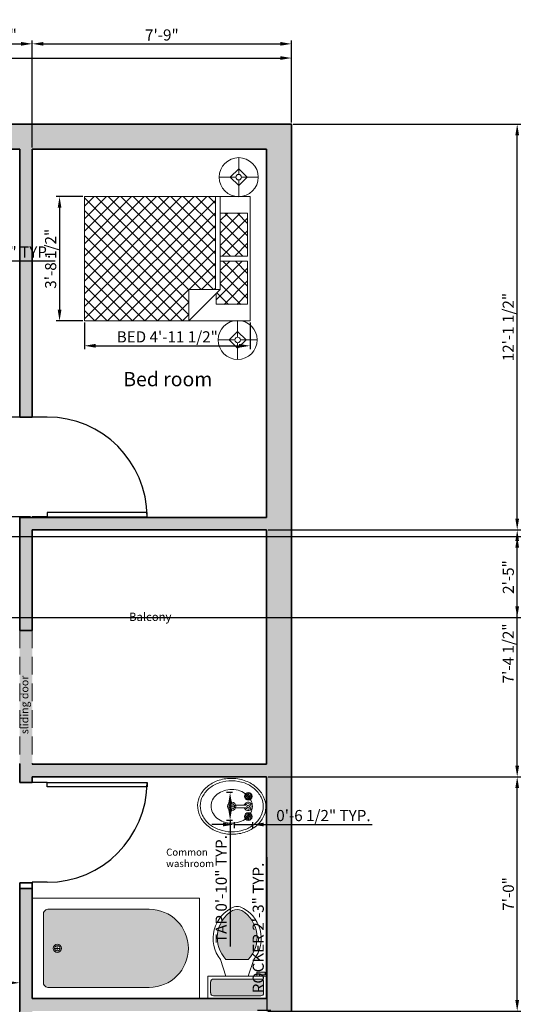
# Model space of a CAD drawing. Units: inches. Extents: x 1872 to 2380, y 714 to 1327.
# Tile 9 of 9: x 2198 to 2380, y 974 to 1327. Entities that reach past the tile are written whole.
import ezdxf

# ---------------------------------------------------------------- set-up
doc = ezdxf.new("R2010")
doc.units = ezdxf.units.IN
doc.linetypes.add('HIDDEN', pattern=[9.525, 6.35, -3.175])
for name, color, linetype, lineweight in [('A-ANNO-DIMS', 2, 'Continuous', 18), ('A-ANNO-TEXT', 7, 'Continuous', 18), ('A-AREA-IDEN', 7, 'Continuous', 18), ('A-DOOR', 4, 'Continuous', 25), ('A-DOOR-HIDN', 4, 'HIDDEN', 18), ('A-FLOR-FIXT', 9, 'Continuous', 20), ('A-FURN', 8, 'Continuous', 18), ('A-WALL', 7, 'Continuous', 35)]:
    doc.layers.add(name, color=color, linetype=linetype, lineweight=lineweight)
for name, color, linetype, lineweight, true_color in [('A-FLOR-FIXT-PATT', 7, 'Continuous', 13, 0xd1ffff), ('A-FURN-PATT', 254, 'Continuous', 13, 0xf8ceb3), ('A-WALL-PATT', 242, 'Continuous', 13, 0xd52e31)]:
    doc.layers.add(name, color=color, linetype=linetype, lineweight=lineweight, true_color=true_color)
doc.styles.get("Standard").update_dxf_attribs({"font": 'arial.ttf'})
doc.dimstyles.new('ISO-25', dxfattribs={"dimtxt": 4, "dimasz": 4, "dimexe": 1.25, "dimexo": 0.625, "dimtad": 1, "dimdec": 0, "dimlunit": 3, "dimtxsty": 'Standard', "dimcen": 2.5, "dimadec": 0, "dimazin": 0, "dimtfac": 1, "dimtdec": 0, "dimtmove": 0, "dimatfit": 3, "dimfxl": 1, "dimarcsym": 0})

# ---------------------------------------------------------------- blocks, each defined once
blk = doc.blocks.new('*U4')
for p, q in [((0, 0), (0, -6)), ((-40, 0), (-40, -6))]:
    blk.add_line(p, q)
blk.add_lwpolyline([(0, 0), (0, 40), (-1.75, 40), (-1.75, 0)], close=True)
blk.add_arc((0, 0), 40, 90, 180)
blk = doc.blocks.new('*U3')
for p, q in [((0, 0), (0, -6)), ((40, 0), (40, -6))]:
    blk.add_line(p, q)
blk.add_lwpolyline([(0, 0), (0, 40), (1.75, 40), (1.75, 0)], close=True)
blk.add_arc((0, 0), 40, 0, 90)
blk = doc.blocks.new('Bed - Queen')
for p, q in [((0, -80.00003), (0, 0)), ((0, 0), (59.99999, 0)), ((59.99999, 0), (59.99999, -80.00003)), ((7.99999, -1.2), (28.79998, -1.2)), ((7.99999, -14.4), (7.99999, -1.2)), ((28.79998, -1.2), (28.79998, -14.4)), ((31.19999, -1.2), (51.99999, -1.2)), ((31.19999, -14.4), (31.19999, -1.2)), ((51.99999, -1.2), (51.99999, -16.4)), ((0, -14.4), (44.8, -14.4)), ((44.8, -16.8), (0, -16.8)), ((59.99999, -29.6), (44.8, -14.4)), ((44.8, -14.4), (44.8, -29.6)), ((51.99999, -16.4), (46.79936, -16.4)), ((44.8, -29.6), (59.99999, -29.6)), ((59.99999, -80.00003), (0, -80.00003))]:
    blk.add_line(p, q)
blk = doc.blocks.new('Lamp - Table')
for p, q in [((0, 7), (0, 1)), ((-1, 0), (-7, 0)), ((0, 3), (-3, 0)), ((-3, 0), (0, -3)), ((3, 0), (0, 3)), ((0, -3), (3, 0)), ((1, 0), (7, 0)), ((0, -1), (0, -7))]:
    blk.add_line(p, q)
for radius in [7, 1]:
    blk.add_circle((0, 0), radius)
blk = doc.blocks.new('Toilet - top')
for p, q in [((9.5, -6), (9.5, -2)), ((-10, -8.5), (-8, -8.5)), ((-10, -9.5), (-10, -8.5)), ((-7, -9.5), (-10, -9.5)), ((-8, -8.5), (-8, -8)), ((-7, -8), (-7, -9.5)), ((-4, -8), (-6, -14)), ((4, -8), (6, -14)), ((4, -14), (-4, -14))]:
    blk.add_line(p, q)
blk.add_lwpolyline([(10.5, -8), (10.5, 0), (-10.5, 0), (-10.5, -8)], close=True)
for points in [[(-9.5, -2), (-9.5, -6)], [(8.5, -1), (-8.5, -1)], [(-8.5, -7), (8.5, -7)]]:
    blk.add_lwpolyline(points)
for centre, radius, start, end in [((-8.62, -1.88), 0.884, 81.8699, 188.1301), ((8.62, -1.88), 0.884, 351.8699, 98.1301), ((-8.62, -6.12), 0.884, 171.8699, 278.1301), ((8.62, -6.12), 0.884, 261.8699, 8.1301), ((3.52, -21.58), 12.17, 141.4691, 247.9714), ((4.2, -21.82), 11.33, 136.3677, 238.9468), ((-3.52, -21.58), 12.17, 292.0284, 38.5307), ((-4.2, -21.82), 11.33, 301.053, 43.6321), ((0, -27.88), 4, 245.7318, 294.2682), ((0, -29), 4, 254.8605, 285.1395)]:
    blk.add_arc(centre, radius, start, end)
blk = doc.blocks.new('Bath Tub - 26 x 60 in.')
for p, q in [((9, -17), (9, -19)), ((8, -18), (10, -18))]:
    blk.add_line(p, q)
blk.add_lwpolyline([(0, -36), (0, 0), (60, 0), (60, -36)], close=True)
for points in [[(4, -30), (4, -6)], [(6, -4), (42, -4)], [(42, -32), (6, -32)]]:
    blk.add_lwpolyline(points)
for radius in [1.5, 1]:
    blk.add_circle((9, -18), radius)
for centre, radius, start, end in [((5.75, -5.75), 1.77, 81.8699, 188.1301), ((42, -18), 14, 270, 90), ((5.75, -30.25), 1.77, 171.8699, 278.1301)]:
    blk.add_arc(centre, radius, start, end)
blk = doc.blocks.new('Sink - Oval top')
for p, q in [((-1, 0), (1, 0)), ((0, 1), (0, -1))]:
    blk.add_line(p, q)
for points in [[(-12.23, 0.39, 0.117634), (-11.46, -3.36, 0.104469), (-8.88, -6.8, 0.090016), (-5.08, -9.07, 0.08192), (-0.32, -10.02, 0.08192), (4.49, -9.38, 0.090016), (8.42, -7.36, 0.104469), (11.22, -4.09, 0.117634), (12.23, -0.39, 0.117634), (11.46, 3.36, 0.104469), (8.88, 6.8, 0.090016), (5.08, 9.07, 0.08192), (0.32, 10.02, 0.08192), (-4.49, 9.38, 0.090016), (-8.42, 7.36, 0.104469), (-11.22, 4.09, 0.117634)], [(-11.29, 0.16, 0.118622), (-10.52, -3.25, 0.104678), (-8.07, -6.36, 0.089562), (-4.54, -8.37, 0.081185), (-0.13, -9.15, 0.081185), (4.3, -8.49, 0.089562), (7.89, -6.58, 0.104678), (10.42, -3.55, 0.118622), (11.29, -0.16, 0.118622), (10.52, 3.25, 0.104678), (8.07, 6.36, 0.089562), (4.54, 8.37, 0.081185), (0.13, 9.15, 0.081185), (-4.3, 8.49, 0.089562), (-7.89, 6.58, 0.104678), (-10.42, 3.55, 0.118622)], [(-7.42, 0.08, 0.118283), (-6.91, -2.17, 0.104607), (-5.29, -4.21, 0.089718), (-2.97, -5.53, 0.081436), (-0.07, -6.04, 0.081436), (2.84, -5.59, 0.089718), (5.2, -4.33, 0.104607), (6.86, -2.32, 0.118283), (7.42, -0.08, 0.118283), (6.91, 2.17, 0.104607), (5.29, 4.21, 0.089718), (2.97, 5.53, 0.081436), (0.07, 6.04, 0.081436), (-2.84, 5.59, 0.089718), (-5.2, 4.33, 0.104607), (-6.86, 2.32, 0.118283)]]:
    blk.add_lwpolyline(points, format="xyb", close=True)
for radius in [1.5, 1]:
    blk.add_circle((0, 0), radius)
blk = doc.blocks.new('Faucet - Bathroom top')
for p, q in [((-4.107, 0.125), (-4.375, 0.125)), ((-3.75, 0.4788), (-3.75, 0.75)), ((-3.5, 0.482), (-3.5, 0.75)), ((-3.1461, 0.125), (-2.875, 0.125)), ((3.143, 0.125), (2.875, 0.125)), ((3.5, 0.4788), (3.5, 0.75)), ((3.75, 0.482), (3.75, 0.75)), ((4.1039, 0.125), (4.375, 0.125)), ((-4.1039, -0.125), (-4.375, -0.125)), ((-3.75, -0.4821), (-3.75, -0.75)), ((-3.5, -0.4789), (-3.5, -0.75)), ((-3.143, -0.125), (-2.875, -0.125)), ((-0.5, -0.8639), (-0.5, -4.5)), ((0.5, -4.5), (0.5, -0.8631)), ((3.1461, -0.125), (2.875, -0.125)), ((3.5, -0.4821), (3.5, -0.75)), ((3.75, -0.4789), (3.75, -0.75)), ((4.107, -0.125), (4.375, -0.125))]:
    blk.add_line(p, q)
for centre, radius in [((-3.625, 0), 1.375), ((-4.625, 0), 0.2795), ((-3.625, 0), 0.5), ((-3.625, 1), 0.2795), ((-2.625, 0), 0.2795), ((0, 0), 0.5), ((3.625, 0), 1.375), ((2.625, 0), 0.2795), ((3.625, 0), 0.5), ((3.625, 1), 0.2795), ((4.625, 0), 0.2795), ((-3.625, -1), 0.2795), ((3.625, -1), 0.2795)]:
    blk.add_circle(centre, radius)
for centre, radius, start, end in [((-3.625, 0), 1, 105.2407, 164.2093), ((-3.625, 0), 1, 16.44125, 74.07887), ((0, 0), 1.5, 289.6514, 250.3603), ((0, 0), 1, 300.3431, 239.7554), ((3.625, 0), 1, 106.12, 164.0884), ((3.625, 0), 1, 16.23422, 73.90469), ((-3.625, 0), 1, 196.2342, 253.9047), ((-3.625, 0), 1, 286.12, 344.0884), ((3.625, 0), 1, 196.4413, 254.0789), ((3.625, 0), 1, 285.2407, 344.2093), ((0, -4.5), 0.5, 180, 0)]:
    blk.add_arc(centre, radius, start, end)
blk = doc.blocks.new('*D22')
at = {"layer": 'A-ANNO-DIMS', "color": 0, "lineweight": -2, "transparency": 16777216}
for p, q in [((1935.4, 1290.27), (1935.4, 1314.61)), ((1939.4, 1313.36), (2291.4, 1313.36)), ((2295.4, 1290.27), (2295.4, 1314.61))]:
    blk.add_line(p, q, dxfattribs=at)
at = {"layer": 'A-ANNO-DIMS', "color": 0, "transparency": 16777216}
for points in [[(1939.4, 1314.03), (1939.4, 1312.69), (1935.4, 1313.36)], [(2291.4, 1314.03), (2291.4, 1312.69), (2295.4, 1313.36)]]:
    blk.add_solid(points, dxfattribs=at)
at = {"layer": 'Defpoints', "color": 0, "transparency": 16777216}
for p in [(2295.4, 1313.36), (1935.4, 1289.64), (2295.4, 1289.64)]:
    blk.add_point(p, dxfattribs=at)
at = {"layer": 'A-ANNO-DIMS', "color": 0, "transparency": 16777216, "insert": (2115.4, 1316.03), "char_height": 4, "attachment_point": 5}
blk.add_mtext("30'", dxfattribs=at)
blk = doc.blocks.new('*D28')
at = {"layer": 'A-ANNO-DIMS', "color": 0, "lineweight": -2, "transparency": 16777216}
for p, q in [((2221.12, 1218.47), (2221.12, 1208.93)), ((2280.56, 1218.47), (2280.56, 1208.93)), ((2225.12, 1210.18), (2276.56, 1210.18))]:
    blk.add_line(p, q, dxfattribs=at)
at = {"layer": 'A-ANNO-DIMS', "color": 0, "transparency": 16777216}
for points in [[(2225.12, 1210.85), (2225.12, 1209.51), (2221.12, 1210.18)], [(2276.56, 1210.85), (2276.56, 1209.51), (2280.56, 1210.18)]]:
    blk.add_solid(points, dxfattribs=at)
at = {"layer": 'Defpoints', "color": 0, "transparency": 16777216}
for p in [(2221.12, 1219.09), (2280.56, 1219.09), (2280.56, 1210.18)]:
    blk.add_point(p, dxfattribs=at)
at = {"layer": 'A-ANNO-DIMS', "color": 0, "transparency": 16777216, "insert": (2250.84, 1212.87), "char_height": 4, "attachment_point": 5}
blk.add_mtext('BED 4\'-11 1/2"', dxfattribs=at)
blk = doc.blocks.new('*D29')
at = {"layer": 'A-ANNO-DIMS', "color": 0, "lineweight": -2, "transparency": 16777216}
for p, q in [((2220.5, 1263.68), (2210.95, 1263.68)), ((2212.2, 1259.68), (2212.2, 1223.09)), ((2220.5, 1219.09), (2210.95, 1219.09))]:
    blk.add_line(p, q, dxfattribs=at)
at = {"layer": 'A-ANNO-DIMS', "color": 0, "transparency": 16777216}
for points in [[(2211.54, 1259.68), (2212.87, 1259.68), (2212.2, 1263.68)], [(2211.54, 1223.09), (2212.87, 1223.09), (2212.2, 1219.09)]]:
    blk.add_solid(points, dxfattribs=at)
at = {"layer": 'Defpoints', "color": 0, "transparency": 16777216}
for p in [(2221.12, 1263.68), (2212.2, 1219.09), (2221.12, 1219.09)]:
    blk.add_point(p, dxfattribs=at)
at = {"layer": 'A-ANNO-DIMS', "color": 0, "transparency": 16777216, "insert": (2209.51, 1241.38), "char_height": 4, "attachment_point": 5, "rotation": 90}
blk.add_mtext('3\'-8 1/2"', dxfattribs=at)
blk = doc.blocks.new('*D32')
at = {"layer": 'A-ANNO-DIMS', "color": 0, "lineweight": -2, "transparency": 16777216}
for p, q in [((2274.25, 1050.03), (2272.12, 1050.03)), ((2273.37, 1046.03), (2273.37, 1044.03)), ((2274.25, 1040.03), (2272.12, 1040.03)), ((2273.37, 1040.03), (2273.37, 994.77))]:
    blk.add_line(p, q, dxfattribs=at)
at = {"layer": 'A-ANNO-DIMS', "color": 0, "transparency": 16777216}
for points in [[(2272.7, 1046.03), (2274.04, 1046.03), (2273.37, 1050.03)], [(2272.7, 1044.03), (2274.04, 1044.03), (2273.37, 1040.03)]]:
    blk.add_solid(points, dxfattribs=at)
at = {"layer": 'Defpoints', "color": 0, "transparency": 16777216}
for p in [(2274.87, 1050.03), (2273.37, 1040.03), (2274.87, 1040.03)]:
    blk.add_point(p, dxfattribs=at)
at = {"layer": 'A-ANNO-DIMS', "color": 0, "transparency": 16777216, "insert": (2270.7, 1015.4), "char_height": 4, "attachment_point": 5, "rotation": 90}
blk.add_mtext('TAP 0\'-10" TYP.', dxfattribs=at)
blk = doc.blocks.new('*D33')
at = {"layer": 'A-ANNO-DIMS', "color": 0, "lineweight": -2, "transparency": 16777216}
for p, q in [((2270.87, 1038.53), (2266.87, 1038.53)), ((2274.87, 1039.41), (2274.87, 1037.28)), ((2274.87, 1038.53), (2281.37, 1038.53)), ((2281.37, 1039.41), (2281.37, 1037.28)), ((2285.37, 1038.53), (2324.32, 1038.53))]:
    blk.add_line(p, q, dxfattribs=at)
at = {"layer": 'A-ANNO-DIMS', "color": 0, "transparency": 16777216}
for points in [[(2270.87, 1039.2), (2270.87, 1037.87), (2274.87, 1038.53)], [(2285.37, 1039.2), (2285.37, 1037.87), (2281.37, 1038.53)]]:
    blk.add_solid(points, dxfattribs=at)
at = {"layer": 'Defpoints', "color": 0, "transparency": 16777216}
for p in [(2274.87, 1040.03), (2281.37, 1040.03), (2281.37, 1038.53)]:
    blk.add_point(p, dxfattribs=at)
at = {"layer": 'A-ANNO-DIMS', "color": 0, "transparency": 16777216, "insert": (2306.85, 1041.23), "char_height": 4, "attachment_point": 5}
blk.add_mtext('0\'-6 1/2" TYP.', dxfattribs=at)
blk = doc.blocks.new('*D36')
at = {"layer": 'A-ANNO-DIMS', "color": 0, "lineweight": -2, "transparency": 16777216}
for p, q in [((2136.87, 1236.27), (2136.87, 1241.85)), ((2140.87, 1240.6), (2165.91, 1240.6)), ((2169.91, 1236.27), (2169.91, 1241.85)), ((2169.91, 1240.6), (2210.57, 1240.6))]:
    blk.add_line(p, q, dxfattribs=at)
at = {"layer": 'A-ANNO-DIMS', "color": 0, "transparency": 16777216}
for points in [[(2140.87, 1241.27), (2140.87, 1239.93), (2136.87, 1240.6)], [(2165.91, 1241.27), (2165.91, 1239.93), (2169.91, 1240.6)]]:
    blk.add_solid(points, dxfattribs=at)
at = {"layer": 'Defpoints', "color": 0, "transparency": 16777216}
for p in [(2169.91, 1240.6), (2136.87, 1235.64), (2169.91, 1235.64)]:
    blk.add_point(p, dxfattribs=at)
at = {"layer": 'A-ANNO-DIMS', "color": 0, "transparency": 16777216, "insert": (2192.24, 1243.29), "char_height": 4, "attachment_point": 5}
blk.add_mtext('WC 2\'-9" TYP.', dxfattribs=at)
blk = doc.blocks.new('*D38')
at = {"layer": 'A-ANNO-DIMS', "color": 0, "lineweight": -2, "transparency": 16777216}
for p, q in [((2286.68, 972), (2286.68, 1026.88)), ((2283.25, 972), (2287.93, 972)), ((2286.68, 949), (2286.68, 968)), ((2283.25, 945), (2287.93, 945))]:
    blk.add_line(p, q, dxfattribs=at)
at = {"layer": 'A-ANNO-DIMS', "color": 0, "transparency": 16777216}
for points in [[(2286.01, 968), (2287.34, 968), (2286.68, 972)], [(2286.01, 949), (2287.34, 949), (2286.68, 945)]]:
    blk.add_solid(points, dxfattribs=at)
at = {"layer": 'Defpoints', "color": 0, "transparency": 16777216}
for p in [(2282.63, 972), (2286.68, 972), (2282.63, 945)]:
    blk.add_point(p, dxfattribs=at)
at = {"layer": 'A-ANNO-DIMS', "color": 0, "transparency": 16777216, "insert": (2283.98, 1001.44), "char_height": 4, "attachment_point": 5, "rotation": 90}
blk.add_mtext('ROCKER 2\'-3" TYP.', dxfattribs=at)
blk = doc.blocks.new('*D54')
at = {"layer": 'A-ANNO-DIMS', "color": 0, "lineweight": -2, "transparency": 16777216}
for p, q in [((2169.91, 1281.27), (2169.91, 1319.69)), ((2173.91, 1318.44), (2198.4, 1318.44)), ((2202.4, 1281.27), (2202.4, 1319.69))]:
    blk.add_line(p, q, dxfattribs=at)
at = {"layer": 'A-ANNO-DIMS', "color": 0, "transparency": 16777216}
for points in [[(2173.91, 1319.11), (2173.91, 1317.78), (2169.91, 1318.44)], [(2198.4, 1319.11), (2198.4, 1317.78), (2202.4, 1318.44)]]:
    blk.add_solid(points, dxfattribs=at)
at = {"layer": 'Defpoints', "color": 0, "transparency": 16777216}
for p in [(2202.4, 1318.44), (2169.91, 1280.64), (2202.4, 1280.64)]:
    blk.add_point(p, dxfattribs=at)
at = {"layer": 'A-ANNO-DIMS', "color": 0, "transparency": 16777216, "insert": (2186.16, 1321.14), "char_height": 4, "attachment_point": 5}
blk.add_mtext('2\'-8 1/2"', dxfattribs=at)
blk = doc.blocks.new('*D55')
at = {"layer": 'A-ANNO-DIMS', "color": 0, "lineweight": -2, "transparency": 16777216}
for p, q in [((2202.4, 1281.27), (2202.4, 1319.69)), ((2206.4, 1318.44), (2291.4, 1318.44)), ((2295.4, 1290.27), (2295.4, 1319.69))]:
    blk.add_line(p, q, dxfattribs=at)
at = {"layer": 'A-ANNO-DIMS', "color": 0, "transparency": 16777216}
for points in [[(2206.4, 1319.11), (2206.4, 1317.78), (2202.4, 1318.44)], [(2291.4, 1319.11), (2291.4, 1317.78), (2295.4, 1318.44)]]:
    blk.add_solid(points, dxfattribs=at)
at = {"layer": 'Defpoints', "color": 0, "transparency": 16777216}
for p in [(2295.4, 1318.44), (2295.4, 1289.64), (2202.4, 1280.64)]:
    blk.add_point(p, dxfattribs=at)
at = {"layer": 'A-ANNO-DIMS', "color": 0, "transparency": 16777216, "insert": (2248.9, 1321.11), "char_height": 4, "attachment_point": 5}
blk.add_mtext('7\'-9"', dxfattribs=at)
blk = doc.blocks.new('*D63')
at = {"layer": 'A-ANNO-DIMS', "color": 0, "lineweight": -2, "transparency": 16777216}
for p, q in [((2287.02, 1055.64), (2377.6, 1055.64)), ((2376.35, 975.64), (2376.35, 1051.64)), ((2287.02, 971.64), (2377.6, 971.64))]:
    blk.add_line(p, q, dxfattribs=at)
at = {"layer": 'A-ANNO-DIMS', "color": 0, "transparency": 16777216}
for points in [[(2375.68, 1051.64), (2377.01, 1051.64), (2376.35, 1055.64)], [(2375.68, 975.64), (2377.01, 975.64), (2376.35, 971.64)]]:
    blk.add_solid(points, dxfattribs=at)
at = {"layer": 'Defpoints', "color": 0, "transparency": 16777216}
for p in [(2286.4, 1055.64), (2376.35, 1055.64), (2286.4, 971.64)]:
    blk.add_point(p, dxfattribs=at)
at = {"layer": 'A-ANNO-DIMS', "color": 0, "transparency": 16777216, "insert": (2373.68, 1013.64), "char_height": 4, "attachment_point": 5, "rotation": 90}
blk.add_mtext('7\'-0"', dxfattribs=at)
blk = doc.blocks.new('*D64')
at = {"layer": 'A-ANNO-DIMS', "color": 0, "lineweight": -2, "transparency": 16777216}
for p, q in [((2287.02, 1144.14), (2377.6, 1144.14)), ((2376.35, 1059.64), (2376.35, 1140.14)), ((2287.02, 1055.64), (2377.6, 1055.64))]:
    blk.add_line(p, q, dxfattribs=at)
at = {"layer": 'A-ANNO-DIMS', "color": 0, "transparency": 16777216}
for points in [[(2375.68, 1140.14), (2377.01, 1140.14), (2376.35, 1144.14)], [(2375.68, 1059.64), (2377.01, 1059.64), (2376.35, 1055.64)]]:
    blk.add_solid(points, dxfattribs=at)
at = {"layer": 'Defpoints', "color": 0, "transparency": 16777216}
for p in [(2286.4, 1144.14), (2376.35, 1144.14), (2286.4, 1055.64)]:
    blk.add_point(p, dxfattribs=at)
at = {"layer": 'A-ANNO-DIMS', "color": 0, "transparency": 16777216, "insert": (2373.65, 1099.89), "char_height": 4, "attachment_point": 5, "rotation": 90}
blk.add_mtext('7\'-4 1/2"', dxfattribs=at)
blk = doc.blocks.new('*D65')
at = {"layer": 'A-ANNO-DIMS', "color": 0, "lineweight": -2, "transparency": 16777216}
for p, q in [((2296.02, 1289.64), (2377.6, 1289.64)), ((2376.35, 1148.14), (2376.35, 1285.64)), ((2287.02, 1144.14), (2377.6, 1144.14))]:
    blk.add_line(p, q, dxfattribs=at)
at = {"layer": 'A-ANNO-DIMS', "color": 0, "transparency": 16777216}
for points in [[(2375.68, 1285.64), (2377.01, 1285.64), (2376.35, 1289.64)], [(2375.68, 1148.14), (2377.01, 1148.14), (2376.35, 1144.14)]]:
    blk.add_solid(points, dxfattribs=at)
at = {"layer": 'Defpoints', "color": 0, "transparency": 16777216}
for p in [(2295.4, 1289.64), (2376.35, 1289.64), (2286.4, 1144.14)]:
    blk.add_point(p, dxfattribs=at)
at = {"layer": 'A-ANNO-DIMS', "color": 0, "transparency": 16777216, "insert": (2373.65, 1216.89), "char_height": 4, "attachment_point": 5, "rotation": 90}
blk.add_mtext('12\'-1 1/2"', dxfattribs=at)
blk = doc.blocks.new('*D69')
at = {"layer": 'A-ANNO-DIMS', "color": 0, "lineweight": -2, "transparency": 16777216}
for p, q in [((2101.02, 1141.77), (2377.6, 1141.77)), ((2376.35, 1116.77), (2376.35, 1137.77)), ((2101.02, 1112.77), (2377.6, 1112.77))]:
    blk.add_line(p, q, dxfattribs=at)
at = {"layer": 'A-ANNO-DIMS', "color": 0, "transparency": 16777216}
for points in [[(2375.68, 1137.77), (2377.01, 1137.77), (2376.35, 1141.77)], [(2375.68, 1116.77), (2377.01, 1116.77), (2376.35, 1112.77)]]:
    blk.add_solid(points, dxfattribs=at)
at = {"layer": 'Defpoints', "color": 0, "transparency": 16777216}
for p in [(2100.4, 1141.77), (2376.35, 1141.77), (2100.4, 1112.77)]:
    blk.add_point(p, dxfattribs=at)
at = {"layer": 'A-ANNO-DIMS', "color": 0, "transparency": 16777216, "insert": (2373.68, 1127.27), "char_height": 4, "attachment_point": 5, "rotation": 90}
blk.add_mtext('2\'-5"', dxfattribs=at)
blk = doc.blocks.new('*D71')
at = {"layer": 'A-ANNO-DIMS', "color": 0, "lineweight": -2, "transparency": 16777216}
for p, q in [((2201.77, 1184.64), (1905.35, 1184.64)), ((1906.6, 1152.84), (1906.6, 1180.64)), ((2201.77, 1148.84), (1905.35, 1148.84))]:
    blk.add_line(p, q, dxfattribs=at)
at = {"layer": 'A-ANNO-DIMS', "color": 0, "transparency": 16777216}
for points in [[(1905.93, 1180.64), (1907.27, 1180.64), (1906.6, 1184.64)], [(1905.93, 1152.84), (1907.27, 1152.84), (1906.6, 1148.84)]]:
    blk.add_solid(points, dxfattribs=at)
at = {"layer": 'Defpoints', "color": 0, "transparency": 16777216}
for p in [(1906.6, 1184.64), (2202.4, 1184.64), (2202.4, 1148.84)]:
    blk.add_point(p, dxfattribs=at)
at = {"layer": 'A-ANNO-DIMS', "color": 0, "transparency": 16777216, "insert": (1903.93, 1166.74), "char_height": 4, "attachment_point": 5, "rotation": 90}
blk.add_mtext('3\'-0"', dxfattribs=at)
blk = doc.blocks.new('*D75')
at = {"layer": 'A-ANNO-DIMS', "color": 0, "lineweight": -2, "transparency": 16777216}
for p, q in [((2166.01, 953.64), (2166.02, 983.06)), ((2170.02, 981.81), (2193.91, 981.8)), ((2197.9, 953.62), (2197.91, 983.04))]:
    blk.add_line(p, q, dxfattribs=at)
at = {"layer": 'A-ANNO-DIMS', "color": 0, "transparency": 16777216}
for points in [[(2170.02, 982.48), (2170.02, 981.14), (2166.02, 981.81)], [(2193.91, 982.46), (2193.91, 981.13), (2197.91, 981.79)]]:
    blk.add_solid(points, dxfattribs=at)
at = {"layer": 'Defpoints', "color": 0, "transparency": 16777216}
for p in [(2197.91, 981.79), (2166.01, 953.01), (2197.9, 952.99)]:
    blk.add_point(p, dxfattribs=at)
at = {"layer": 'A-ANNO-DIMS', "color": 0, "transparency": 16777216, "insert": (2181.97, 984.47), "char_height": 4, "attachment_point": 5, "rotation": 359.9714}
blk.add_mtext('2\'-8"', dxfattribs=at)

msp = doc.modelspace()

# ---------------------------------------------------------------- hatches: boundary and pattern name
at = {"layer": 'A-FLOR-FIXT-PATT', "transparency": 33554687}
h = msp.add_hatch(color=256, dxfattribs=at)
h.dxf.hatch_style = 1
h.paths.add_polyline_path([(2244.4, 1008.14), (2208.4, 1008.14, 0.5), (2206.4, 1006.14), (2206.4, 982.14, 0.5), (2208.4, 980.14), (2244.4, 980.14, 1)])
h.paths.add_polyline_path([(2209.9, 994.14, -1), (2212.9, 994.14, -1)], flags=16)
h.paths.add_polyline_path([(2210.4, 994.14, -1), (2212.4, 994.14, -1)], flags=0)
h.paths.add_polyline_path([(2151.91, 1276.64), (2115.91, 1276.64, 0.5), (2113.91, 1274.64), (2113.91, 1250.64, 0.5), (2115.91, 1248.64), (2151.91, 1248.64, 1)])
h.paths.add_polyline_path([(2117.41, 1262.64, -1), (2120.41, 1262.64, -1)], flags=16)
h.paths.add_polyline_path([(2117.91, 1262.64, -1), (2119.91, 1262.64, -1)], flags=0)
h = msp.add_hatch(color=256, dxfattribs=at)
h.dxf.hatch_style = 1
h.paths.add_polyline_path([(2155.91, 1229.14, 0.48008), (2138.39, 1226.79, 0.215004), (2138.39, 1223.5, 0.48008), (2155.91, 1221.14)])
h.paths.add_polyline_path([(2168.91, 1233.64, 0.5), (2167.91, 1234.64), (2163.91, 1234.64, 0.5), (2162.91, 1233.64), (2162.91, 1216.64, 0.5), (2163.91, 1215.64), (2167.91, 1215.64, 0.5), (2168.91, 1216.64)])
h.paths.add_polyline_path([(2285.4, 982.14, 0.5), (2284.4, 983.14), (2267.4, 983.14, 0.5), (2266.4, 982.14), (2266.4, 978.14, 0.5), (2267.4, 977.14), (2284.4, 977.14, 0.5), (2285.4, 978.14)])
h.paths.add_polyline_path([(2277.54, 1007.66, 0.215004), (2274.25, 1007.66, 0.48008), (2271.9, 990.14), (2279.9, 990.14, 0.48008)])
h.paths.add_polyline_path([(2285.9, 985.64), (2282.9, 985.64), (2282.9, 984.14), (2283.9, 984.14), (2283.9, 984.64), (2285.9, 984.64)])
h.paths.add_polyline_path([(2279.53, 1049.02, -0.039819), (2280.2, 1048.28, 0.216904), (2280.37, 1048.66, 0.658258)])
h.paths.add_polyline_path([(2279.53, 1049.02, 0.206085), (2279.37, 1048.66, 0.643515), (2280.2, 1048.28, 0.039819)])
h.paths.add_polyline_path([(2279.37, 1045.03, 1), (2280.37, 1045.03, 1)])
h.paths.add_polyline_path([(2280.37, 1041.41, 0.219955), (2280.19, 1041.79, -0.039801), (2279.52, 1041.05, 0.66578)])
h.paths.add_polyline_path([(2280.19, 1041.79, 0.639405), (2279.37, 1041.41, 0.200639), (2279.52, 1041.05, 0.039801)])
h.paths.add_polyline_path([(2158.34, 1154.61, 1), (2157.34, 1154.61, 1)])
h.paths.add_polyline_path([(2154.72, 1154.61, 1), (2153.72, 1154.61, 1)])
h.paths.add_polyline_path([(2161.97, 1154.61, 1), (2160.97, 1154.61, 1)])
h.paths.add_polyline_path([(2180.69, 824, 1), (2181.69, 824, 1)])
h.paths.add_polyline_path([(2185.32, 824, 1), (2184.32, 824, 1)])
h.paths.add_polyline_path([(2188.94, 824, 1), (2187.94, 824, 1)])
at = {"layer": 'A-FURN-PATT', "transparency": 33554687}
h = msp.add_hatch(dxfattribs=at)
h.set_pattern_fill('ANSI37', color=256)
h.paths.add_polyline_path([(2030.37, 1262.04), (1979.97, 1262.04), (1979.97, 1246.84), (1967.17, 1246.84), (1967.17, 1202.04), (2030.37, 1202.04)])
h.paths.add_polyline_path([(1964.77, 1246.84), (1966.77, 1248.84), (1966.77, 1254.04), (1951.57, 1254.04), (1951.57, 1233.24), (1964.77, 1233.24)])
h.paths.add_polyline_path([(1964.77, 1230.84), (1951.57, 1230.84), (1951.57, 1210.04), (1964.77, 1210.04)])
h.paths.add_polyline_path([(2268.08, 1263.68), (2221.12, 1263.68), (2221.12, 1219.09), (2258.57, 1219.09), (2258.57, 1230.39), (2268.08, 1230.39)])
h.paths.add_polyline_path([(2279.67, 1257.73), (2269.86, 1257.73), (2269.86, 1242.28), (2279.67, 1242.28)])
h.paths.add_polyline_path([(2279.67, 1240.49), (2269.86, 1240.49), (2269.86, 1230.39), (2268.38, 1228.9), (2268.38, 1225.04), (2279.67, 1225.04)])
h.paths.add_polyline_path([(2097.97, 1011.83), (2085.54, 1011.83), (2085.42, 1011.06), (2098.09, 1011.06)])
h.paths.add_polyline_path([(2098.15, 1010.67), (2085.36, 1010.67), (2084.39, 1004.45), (2099.13, 1004.45)])
h.paths.add_polyline_path([(2119.91, 1010.67), (2107.12, 1010.67), (2106.14, 1004.45), (2120.89, 1004.45)])
h.paths.add_polyline_path([(2119.73, 1011.83), (2107.3, 1011.83), (2107.18, 1011.06), (2119.85, 1011.06)])
h.paths.add_polyline_path([(2074.66, 997.83), (2068.44, 996.86), (2068.44, 984.06), (2074.66, 983.09)])
h.paths.add_polyline_path([(2068.05, 996.8), (2067.28, 996.68), (2067.28, 984.25), (2068.05, 984.12)])
h.paths.add_polyline_path([(2136.83, 996.86), (2130.61, 997.83), (2130.61, 983.09), (2136.83, 984.06)])
h.paths.add_polyline_path([(2137.99, 996.68), (2137.22, 996.8), (2137.22, 984.12), (2137.99, 984.25)])
h.paths.add_polyline_path([(2099.13, 976.47), (2084.39, 976.47), (2085.36, 970.26), (2098.15, 970.26)])
h.paths.add_polyline_path([(2120.89, 976.47), (2106.14, 976.47), (2107.12, 970.26), (2119.91, 970.26)])
h.paths.add_polyline_path([(2119.85, 969.87), (2107.18, 969.87), (2107.3, 969.09), (2119.73, 969.09)])
h.paths.add_polyline_path([(2098.09, 969.87), (2085.42, 969.87), (2085.54, 969.09), (2097.97, 969.09)])
at = {"layer": 'A-WALL-PATT', "transparency": 33554687}
h = msp.add_hatch(color=256, dxfattribs=at)
h.dxf.hatch_style = 1
h.paths.add_polyline_path([(2295.4, 1289.64), (1935.4, 1289.64), (1935.4, 809.64), (1949.4, 809.64), (1949.4, 818.64), (1944.4, 818.64), (1944.4, 1108.27), (2100.4, 1108.27), (2100.4, 1112.77), (1944.4, 1112.77), (1944.4, 1280.64), (2095.9, 1280.64), (2095.9, 1141.77), (2100.4, 1141.77), (2100.4, 1280.64), (2169.91, 1280.64), (2169.91, 1244.64), (2169.91, 1160.49, -0.053008), (2170.04, 1158.75, -0.03687), (2169.91, 1157.54), (2169.91, 1148.64), (2167.91, 1148.64), (2138.4, 1148.64), (2138.4, 1144.14), (2167.91, 1144.14), (2174.41, 1144.14), (2174.41, 1280.64), (2197.9, 1280.64), (2197.9, 1184.64), (2202.4, 1184.64), (2202.4, 1280.64), (2286.4, 1280.64), (2286.4, 1148.64), (2197.9, 1148.64), (2197.9, 1108.14), (2202.4, 1108.14), (2202.4, 1144.14), (2286.4, 1144.14), (2286.4, 1060.14), (2202.4, 1060.14), (2202.4, 1108.14), (2197.9, 1108.14), (2197.9, 1060.14), (2197.9, 1053.64), (2202.4, 1053.64), (2202.4, 1055.64), (2286.4, 1055.64), (2286.4, 976.14), (2202.4, 976.14), (2202.4, 1015.64), (2197.9, 1015.64), (2197.9, 971.64), (2197.9, 952.99), (2197.9, 818.64), (2101.9, 818.64), (2101.9, 948.71), (2130.4, 948.71), (2130.4, 952.99), (2073.4, 952.99), (2073.4, 948.71), (2097.4, 948.71), (2097.4, 818.64), (2005.9, 818.64), (2005.9, 948.71), (2029.9, 948.71), (2029.9, 952.99), (2001.4, 952.99), (2001.4, 818.64), (1996.4, 818.64), (1985.23, 818.64), (1985.23, 809.64), (1996.4, 809.64), (2295.4, 809.64)])
h.paths.add_polyline_path([(2202.4, 971.64), (2286.4, 971.64), (2286.4, 858.19), (2286.62, 858.19), (2286.62, 857.19), (2286.4, 857.19), (2286.4, 828.68), (2286.48, 828.76), (2286.4, 828.43), (2286.4, 818.64), (2256.29, 818.64), (2255.29, 818.39), (2254.54, 818.64), (2238.99, 818.64), (2238.75, 818.58), (2238.56, 818.64), (2202.4, 818.64), (2202.4, 952.99)], flags=16)
h.paths.add_polyline_path([(2260.41, 970, -0.15), (2280.41, 970), (2278.41, 967, 0.001913), (2277.92, 967.06), (2277.41, 964.5), (2278.64, 964.5), (2278.72, 964), (2279.41, 964), (2282.41, 953, -0.541163), (2280.76, 950.93), (2280.91, 950, -0.414214), (2279.91, 949), (2279.41, 949), (2279.91, 945), (2278.41, 945), (2277.91, 949), (2270.41, 949), (2262.91, 949), (2262.41, 945), (2260.91, 945), (2261.41, 949), (2260.91, 949, -0.414214), (2259.91, 950), (2260.05, 950.93, -0.505809), (2258.36, 952.83), (2261.41, 964), (2262.1, 964), (2262.17, 964.5), (2263.41, 964.5), (2262.9, 967.06, 0.001913), (2262.41, 967)], flags=0)
h.paths.add_polyline_path([(2257.85, 934.42), (2280.51, 934.42, -0.333333), (2281.77, 933.16), (2281.77, 923.09, -0.333333), (2280.51, 921.83), (2277.57, 921.83), (2277.57, 921.41), (2275.89, 921.41), (2275.89, 921.83), (2262.46, 921.83), (2262.46, 921.41), (2260.79, 921.41), (2260.79, 921.83), (2257.85, 921.83, -0.333333), (2256.59, 923.09), (2256.59, 933.16, -0.333333)], flags=0)
h.paths.add_polyline_path([(2260.61, 912.79), (2262.11, 912.79), (2262.61, 908.79), (2270.11, 908.79), (2277.61, 908.79), (2278.11, 912.79), (2279.61, 912.79), (2279.11, 908.79), (2279.61, 908.79, -0.414214), (2280.61, 907.79), (2280.46, 906.86, -0.505809), (2282.15, 904.96), (2279.11, 893.79), (2278.42, 893.79), (2278.34, 893.29), (2277.11, 893.29), (2277.62, 890.73, 0.001913), (2278.11, 890.79), (2280.11, 887.79, -0.15), (2260.11, 887.79), (2262.11, 890.79, 0.001913), (2262.59, 890.73), (2263.11, 893.29), (2261.87, 893.29), (2261.79, 893.79), (2261.11, 893.79), (2258.11, 904.79, -0.541163), (2259.75, 906.86), (2259.61, 907.79, -0.414214), (2260.61, 908.79), (2261.11, 908.79)], flags=0)
h.paths.add_polyline_path([(2252.62, 864.69), (2253.62, 864.69), (2253.62, 862.19), (2253.62, 860.69), (2256.62, 859.69, -0.362186), (2259.62, 862.19, -0.174416), (2262.62, 860.69, 0.103487), (2265.62, 859.19, -0.219276), (2266.55, 858.19), (2268.62, 858.19), (2268.62, 859.69), (2267.62, 859.69), (2267.62, 863.69), (2270.12, 863.69), (2270.12, 859.69), (2269.12, 859.69), (2269.12, 858.19), (2274.62, 858.19), (2278.62, 858.19), (2278.62, 862.69), (2275.62, 864.69), (2275.62, 865.69), (2279.62, 862.69), (2279.62, 858.19), (2279.62, 852.69), (2275.62, 849.19), (2275.62, 850.19), (2278.62, 852.69), (2278.62, 857.19), (2274.62, 857.19), (2271.12, 857.19), (2271.12, 855.69), (2272.12, 855.69), (2272.12, 851.69), (2269.62, 851.69), (2269.62, 855.69), (2270.62, 855.69), (2270.62, 857.19), (2266.55, 857.19, -0.219162), (2265.62, 856.19, 0.103506), (2262.62, 854.69, -0.174459), (2259.62, 853.19, -0.362114), (2256.62, 855.69), (2253.62, 854.69), (2253.62, 850.69), (2252.62, 850.69)], flags=0)
h.paths.add_polyline_path([(2253.62, 859.69), (2256.62, 858.69), (2256.62, 856.69), (2253.62, 855.69)], flags=0)
h.paths.add_polyline_path([(2208.62, 838.17), (2208.28, 836.61), (2207.75, 836.18), (2207.67, 833.93), (2208.71, 832.96), (2211.55, 836.09), (2214.43, 837.53), (2214.45, 837.55), (2214.61, 836.16), (2215.48, 834.9), (2215.87, 835.13), (2217.12, 836.79), (2216.83, 834.17), (2218.8, 828.76), (2219.23, 829.13), (2220.06, 831.53), (2219.5, 837.61), (2219.53, 837.66), (2219.68, 838.72), (2219.62, 838.91), (2219.72, 839.01), (2219.51, 837.47), (2219.77, 834.68), (2220.87, 834.05), (2221.03, 834.58), (2222.05, 835.47), (2222.71, 834.65), (2223.67, 836.89), (2224.63, 836.57), (2226.23, 835.08), (2227.55, 836.18), (2227.59, 837.16), (2228.42, 838.17), (2228.08, 836.61), (2227.55, 836.18), (2227.47, 833.93), (2228.51, 832.96), (2231.35, 836.09), (2234.23, 837.53), (2234.25, 837.55), (2234.42, 836.16), (2235.28, 834.9), (2235.67, 835.13), (2236.93, 836.79), (2236.93, 836.84), (2238.69, 834.65), (2239.41, 836.34), (2239.3, 837.61), (2239.34, 837.66), (2239.48, 838.72), (2239.42, 838.91), (2239.52, 839.01), (2239.31, 837.47), (2239.36, 836.98), (2240.61, 836.57), (2242.2, 835.08), (2243.53, 836.18), (2243.57, 837.16), (2244.39, 838.17), (2244.05, 836.61), (2243.53, 836.18), (2243.44, 833.93), (2244.49, 832.96), (2247.33, 836.09), (2250.21, 837.53), (2250.22, 837.55), (2250.39, 836.16), (2251.25, 834.9), (2251.65, 835.13), (2252.9, 836.79), (2252.61, 834.17), (2254.09, 830.08), (2254.54, 829.37), (2254.85, 828.99), (2255.01, 829.13), (2255.83, 831.53), (2255.29, 837.44), (2255.28, 837.44), (2255.46, 838.72), (2255.4, 838.91), (2255.5, 839.01), (2255.28, 837.47), (2255.29, 837.44), (2257.9, 836.57), (2259.5, 835.08), (2260.82, 836.18), (2260.86, 837.16), (2261.69, 838.17), (2261.35, 836.61), (2260.82, 836.18), (2260.74, 833.93), (2261.78, 832.96), (2264.62, 836.09), (2267.5, 837.53), (2267.52, 837.55), (2267.68, 836.16), (2268.54, 834.9), (2268.94, 835.13), (2270.19, 836.79), (2269.9, 834.17), (2271.79, 828.96), (2271.98, 828.86), (2272.3, 829.13), (2273.13, 831.53), (2272.56, 837.61), (2272.6, 837.66), (2272.75, 838.72), (2272.69, 838.91), (2272.79, 839.01), (2272.58, 837.47), (2273.13, 831.53), (2273.02, 831.22), (2273.67, 831.01), (2273.92, 831.6), (2273.83, 830.95), (2274.1, 830.86), (2275.75, 833.35), (2276.03, 831.86), (2276.57, 831.38), (2277, 831.91), (2277.3, 833.27), (2279.06, 830.44), (2281.09, 831.46), (2281.1, 831.48), (2281.21, 830.5), (2281.82, 829.61), (2282.1, 829.77), (2282.98, 830.94), (2282.77, 829.1), (2284.15, 825.3), (2284.46, 825.55), (2285.04, 827.24), (2284.64, 831.51), (2284.67, 831.55), (2284.77, 832.3), (2284.73, 832.43), (2284.8, 832.5), (2284.65, 831.42), (2285.04, 827.24), (2284.46, 825.55), (2283.45, 824.71), (2281.76, 819.99), (2278.73, 818.64), (2276.7, 819.65), (2275.69, 821.34), (2274.34, 822.01), (2272.32, 824.04), (2269.58, 824.33), (2268.46, 821.21), (2264.14, 819.29), (2261.26, 820.73), (2259.82, 823.13), (2257.9, 824.09), (2255.02, 826.97), (2253.29, 827.15), (2251.17, 821.21), (2246.85, 819.29), (2243.97, 820.73), (2242.53, 823.13), (2240.61, 824.09), (2237.73, 826.97), (2237.27, 827.01), (2235.19, 821.21), (2230.87, 819.29), (2227.99, 820.73), (2226.55, 823.13), (2224.63, 824.09), (2221.75, 826.97), (2217.61, 827.41), (2215.39, 821.21), (2211.07, 819.29), (2208.19, 820.73), (2206.75, 823.13), (2204.83, 824.09), (2203.87, 826.49), (2202.91, 830.81), (2202.91, 834.65), (2203.87, 836.89), (2204.83, 836.57), (2206.43, 835.08), (2207.75, 836.18), (2207.79, 837.16)], flags=0)
h.paths.add_polyline_path([(2221.04, 832.88), (2221.82, 832.52), (2222.11, 833.69), (2222.71, 834.29), (2222.71, 832.11), (2225.59, 830.81), (2226.55, 830.81), (2228.95, 822.65), (2230.87, 820.25), (2230.87, 819.29), (2233.27, 821.21), (2233.75, 823.61), (2232.79, 826.97), (2231.99, 830.19), (2236.41, 827.71), (2236.63, 831.29), (2235.93, 834.58), (2242.53, 830.81), (2241.57, 830.81), (2240.97, 831.07), (2240.47, 830.33), (2239.06, 829.14), (2239.65, 826.49), (2237.25, 829.37), (2236.52, 829.55), (2236.41, 827.71), (2231.99, 830.19), (2232.79, 826.97), (2233.75, 823.61), (2233.27, 821.21), (2230.87, 819.29), (2230.87, 820.25), (2228.95, 822.65), (2226.55, 830.81), (2225.59, 830.81), (2222.71, 832.11), (2222.71, 830.81), (2223.67, 826.49), (2221.27, 829.37), (2220.67, 830.33), (2220.67, 830.33)], flags=0)
h.paths.add_polyline_path([(2255.98, 833), (2259.82, 830.81), (2258.86, 830.81), (2257.25, 831.54), (2256.45, 830.33), (2256.66, 831.81), (2256.02, 832.1), (2255.98, 831.99)], flags=0)
h.paths.add_polyline_path([(2275.69, 826.73), (2277.07, 828.25), (2275.46, 829.74), (2276.39, 830.51), (2276.33, 828.93), (2279.06, 826.4), (2278.73, 823.36), (2277.38, 821)], flags=0)
h.paths.add_polyline_path([(2260.6, 925.25), (2276.34, 925.25), (2276.34, 931.01), (2260.6, 931.01)], flags=8)
h.paths.add_polyline_path([(2202.72, 1070.05), (2202.72, 1092.72), (2197.34, 1092.72), (2197.34, 1070.05)], flags=25)

# ---------------------------------------------------------------- linework, layer by layer
at = {"layer": 'A-DOOR-HIDN', "transparency": 33554687}
for p, q in [((2197.9, 1108.14), (2197.9, 1060.14)), ((2202.4, 1108.14), (2202.4, 1060.14))]:
    msp.add_line(p, q, dxfattribs=at)
at = {"layer": 'A-WALL', "transparency": 33554687}
for p, q in [((2174.41, 1280.64), (2197.9, 1280.64)), ((2202.4, 1280.64), (2286.4, 1280.64)), ((2286.4, 1144.14), (2286.4, 1060.14)), ((2286.4, 1055.64), (2286.4, 976.14)), ((2197.9, 1053.64), (2202.4, 1053.64)), ((2197.9, 1017.64), (2202.4, 1017.64)), ((2197.9, 1017.64), (2197.9, 971.64)), ((2202.4, 1017.64), (2202.4, 976.14)), ((2197.9, 1015.64), (2202.4, 1015.64))]:
    msp.add_line(p, q, dxfattribs=at)
at = {"layer": 'A-WALL'}
for p, q in [((2197.9, 1280.64), (2197.9, 1184.64)), ((2202.4, 1280.64), (2202.4, 1184.64)), ((2286.4, 1280.64), (2286.4, 1148.64)), ((2197.9, 1184.64), (2202.4, 1184.64)), ((2197.9, 1148.64), (2286.4, 1148.64)), ((2197.9, 1148.64), (2197.9, 1108.14)), ((2202.4, 1144.14), (2286.4, 1144.14)), ((2202.4, 1144.14), (2202.4, 1108.14)), ((2197.9, 1108.14), (2202.4, 1108.14)), ((2197.9, 1060.14), (2197.9, 1053.64)), ((2202.4, 1060.14), (2286.4, 1060.14)), ((2202.4, 1055.64), (2286.4, 1055.64)), ((2202.4, 1055.64), (2202.4, 1053.64)), ((2202.4, 976.14), (2286.4, 976.14))]:
    msp.add_line(p, q, dxfattribs=at)
at = {"layer": 'A-WALL', "transparency": 33554687}
msp.add_lwpolyline([(1949.4, 809.64), (1935.4, 809.64), (1935.4, 1289.64), (2295.4, 1289.64), (2295.4, 809.64), (1996.4, 809.64)], dxfattribs=at)

# ---------------------------------------------------------------- block references
at = {"layer": 'A-DOOR', "xscale": 0.895133583936691, "yscale": 0.895133583936691, "zscale": 0.895133583936691, "rotation": 270}
msp.add_blockref('*U4', (2207.77, 1148.84), dxfattribs=at)
at = {"layer": 'A-DOOR', "transparency": 33554687, "xscale": 0.895133583936691, "yscale": 0.895133583936691, "zscale": 0.895133583936691, "rotation": 270}
msp.add_blockref('*U3', (2207.77, 1053.64), dxfattribs=at)
at = {"layer": 'A-FLOR-FIXT', "transparency": 33554687}
for name, p in [('Sink - Oval top', (2273.95, 1045.06)), ('Bath Tub - 26 x 60 in.', (2202.4, 1012.14))]:
    msp.add_blockref(name, p, dxfattribs=at)
for name, p, rotation in [('Faucet - Bathroom top', (2279.87, 1045.03), 270), ('Toilet - top', (2275.9, 976.14), 180)]:
    msp.add_blockref(name, p, dxfattribs=dict(at, rotation=rotation))
at = {"layer": 'A-FURN', "transparency": 33554687}
for p in [(2276.45, 1270.63), (2276.08, 1212.28)]:
    msp.add_blockref('Lamp - Table', p, dxfattribs=at)
at = {"layer": 'A-FURN', "transparency": 33554687, "xscale": 0.7430096615388373, "yscale": 0.7430096615388373, "zscale": 0.7430096615388373, "rotation": 270}
msp.add_blockref('Bed - Queen', (2280.56, 1263.68), dxfattribs=at)

# ---------------------------------------------------------------- texts
at = {"layer": 'A-ANNO-TEXT', "transparency": 33554687}
msp.add_text('sliding door ', height=2.7718, rotation=90, dxfattribs=at).set_placement((2201.01, 1070.95))
at = {"layer": 'A-AREA-IDEN', "transparency": 33554687}
for s, height, p in [('Bed room ', 5.107, (2235.06, 1195.67)), ('Balcony', 2.965, (2237.14, 1111.52)), ('Common ', 2.541, (2250.43, 1027.35)), ('washroom', 2.541, (2250.43, 1023.27))]:
    msp.add_text(s, height=height, dxfattribs=at).set_placement(p)

# ---------------------------------------------------------------- dimensions: what is measured, and where the dimension line sits
at = {"layer": 'A-ANNO-DIMS', "transparency": 33554687}
for base, p1, p2, override, picture, middle in [((2202.4, 1318.44), (2169.91, 1280.64), (2202.4, 1280.64), {"dimdec": 1, "dimlfac": 1, "dimrnd": 0, "dimzin": 1, "dimdsep": 46, "dimlunit": 4, "dimfrac": 2}, '*D54', (2186.16, 1321.14)), ((2295.4, 1318.44), (2202.4, 1280.64), (2295.4, 1289.64), {"dimdec": 1, "dimlfac": 1, "dimrnd": 0, "dimzin": 1, "dimdsep": 46, "dimlunit": 4, "dimfrac": 2}, '*D55', (2248.9, 1321.11)), ((2295.4, 1313.36), (1935.4, 1289.64), (2295.4, 1289.64), {"dimclrd": 0, "dimclre": 0, "dimclrt": 0}, '*D22', (2115.4, 1316.03))]:
    dim = msp.add_linear_dim(base=base, p1=p1, p2=p2, dimstyle='ISO-25', override=override, dxfattribs=at)
    dim.commit()
    dim.dimension.update_dxf_attribs({"geometry": picture, "text_midpoint": middle})
for base, p1, p2, angle, picture, middle in [((2376.35, 1289.64), (2286.4, 1144.14), (2295.4, 1289.64), 90, '*D65', (2373.65, 1216.89)), ((2212.2, 1219.09), (2221.12, 1263.68), (2221.12, 1219.09), 270, '*D29', (2209.51, 1241.38)), ((1906.6, 1184.64), (2202.4, 1148.84), (2202.4, 1184.64), 90, '*D71', (1903.93, 1166.74)), ((2376.35, 1144.14), (2286.4, 1055.64), (2286.4, 1144.14), 90, '*D64', (2373.65, 1099.89)), ((2376.35, 1141.77), (2100.4, 1112.77), (2100.4, 1141.77), 90, '*D69', (2373.68, 1127.27)), ((2376.35, 1055.64), (2286.4, 971.64), (2286.4, 1055.64), 90, '*D63', (2373.68, 1013.64)), ((2197.91, 981.79), (2166.01, 953.01), (2197.9, 952.99), 359.9714, '*D75', (2181.97, 984.47))]:
    dim = msp.add_linear_dim(base=base, p1=p1, p2=p2, angle=angle, dimstyle='ISO-25', override={"dimdec": 1, "dimlfac": 1, "dimrnd": 0, "dimzin": 1, "dimdsep": 46, "dimlunit": 4, "dimfrac": 2}, dxfattribs=at)
    dim.commit()
    dim.dimension.update_dxf_attribs({"geometry": picture, "text_midpoint": middle})
for base, p1, p2, text, picture, middle in [((2169.91, 1240.6), (2136.87, 1235.64), (2169.91, 1235.64), 'WC <> TYP.', '*D36', (2192.24, 1243.29)), ((2280.56, 1210.18), (2221.12, 1219.09), (2280.56, 1219.09), 'BED <>', '*D28', (2250.84, 1212.87)), ((2281.37, 1038.53), (2274.87, 1040.03), (2281.37, 1040.03), '<> TYP.', '*D33', (2306.85, 1041.23))]:
    dim = msp.add_linear_dim(base=base, p1=p1, p2=p2, text=text, dimstyle='ISO-25', override={"dimdec": 1, "dimlfac": 1, "dimrnd": 0, "dimzin": 1, "dimdsep": 46, "dimlunit": 4, "dimfrac": 2}, dxfattribs=at)
    dim.commit()
    dim.dimension.update_dxf_attribs({"geometry": picture, "text_midpoint": middle})
for base, p1, p2, angle, text, picture, middle in [((2273.37, 1040.03), (2274.87, 1050.03), (2274.87, 1040.03), 270, 'TAP <> TYP.', '*D32', (2270.7, 1015.4)), ((2286.68, 972), (2282.63, 945), (2282.63, 972), 90, 'ROCKER <> TYP.', '*D38', (2283.98, 1001.44))]:
    dim = msp.add_linear_dim(base=base, p1=p1, p2=p2, angle=angle, text=text, dimstyle='ISO-25', override={"dimdec": 1, "dimlfac": 1, "dimrnd": 0, "dimzin": 1, "dimdsep": 46, "dimlunit": 4, "dimfrac": 2}, dxfattribs=at)
    dim.commit()
    dim.dimension.update_dxf_attribs({"geometry": picture, "text_midpoint": middle})

doc.saveas('drawing.dxf')
